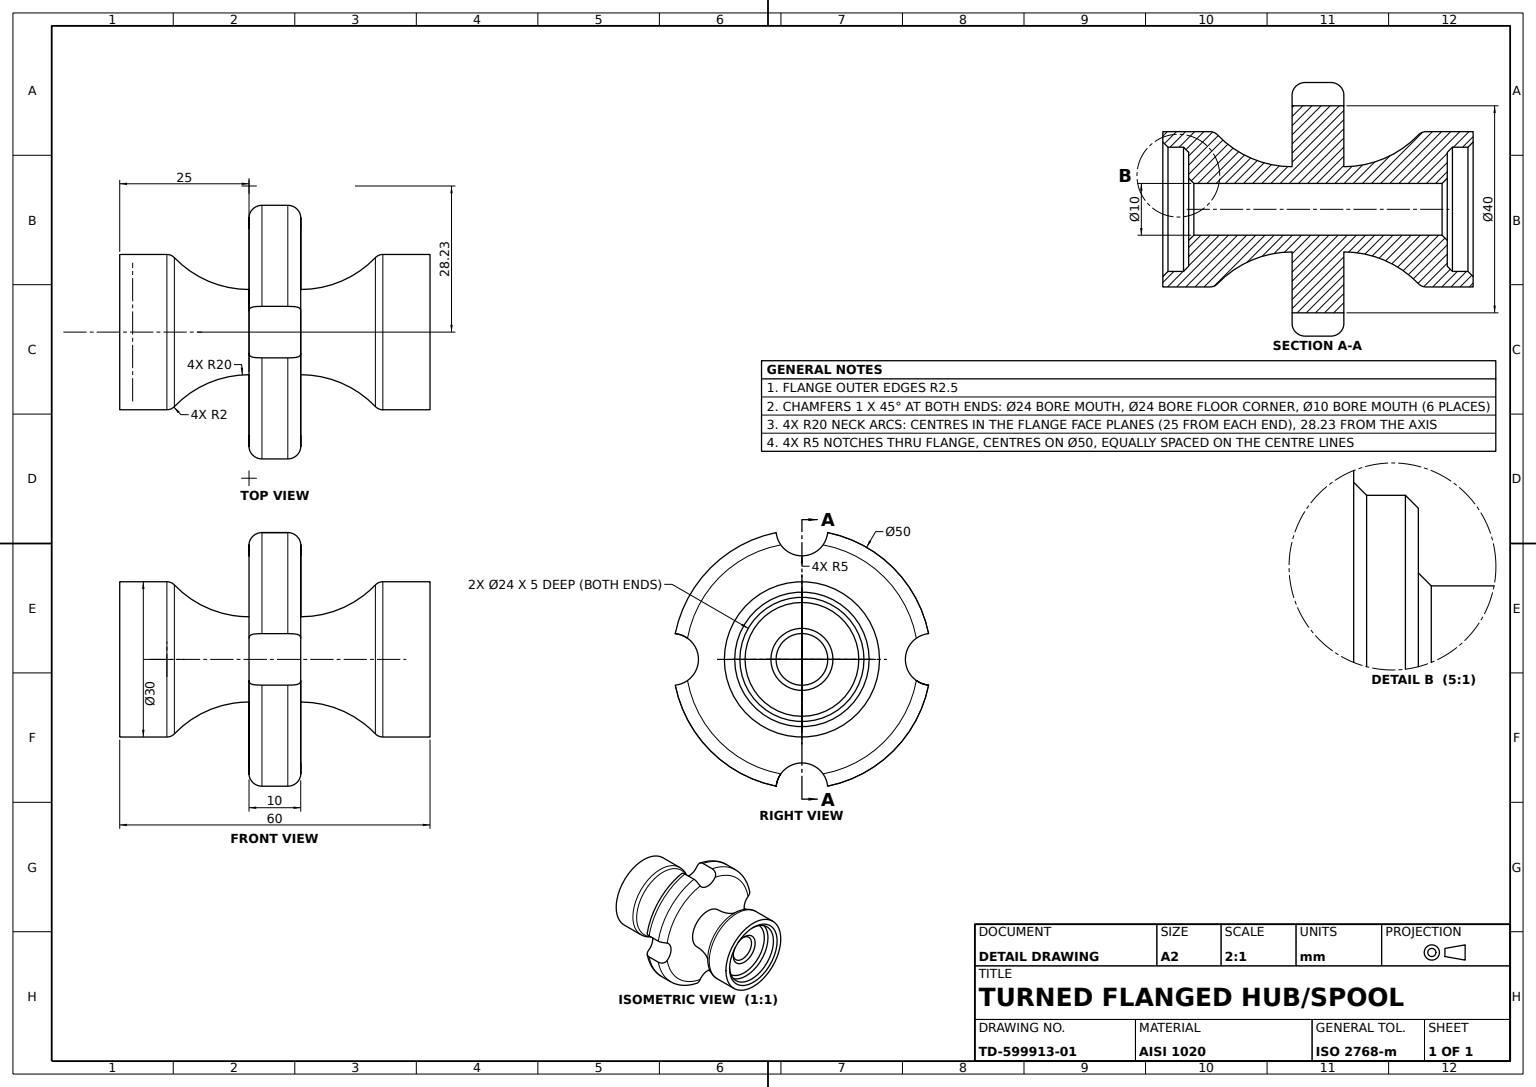
from build123d import *

# Parameters (mm, degrees)
FLANGE_FILLET_R2_5_R     = 2.5
FLANGE_NOTCHES_4X_REACH  = 51.749
FLANGE_NOTCH_SKETCH_R    = 5
EDGE_CHAMFER_1X45_A_SIZE = 1
EDGE_FILLET_R2_R         = 2
EDGE_CHAMFER_1X45_B_SIZE = 1


with BuildPart() as part:
    # Hub Profile Sketch → Hub Body Revolve (revolve)
    with BuildSketch(Plane.XY, mode=Mode.PRIVATE) as hub_body_revolve_sk:
        with BuildLine():
            Line((12, 0), (12, 5))
            Line((12, 5), (5, 5))
            Line((5, 5), (5, 55))
            Line((5, 55), (12, 55))
            Line((12, 55), (12, 60))
            Line((12, 60), (15, 60))
            Line((15, 60), (15, 50))
            ThreePointArc((15, 50), (10, 43.228756555), (8.228756555, 35))
            Line((8.228756555, 35), (25, 35))
            Line((25, 35), (25, 25))
            Line((25, 25), (8.228756555, 25))
            ThreePointArc((8.228756555, 25), (10, 16.771243445), (15, 10))
            Line((15, 10), (15, 0))
            Line((15, 0), (12, 0))
        make_face()
    revolve(hub_body_revolve_sk.sketch.rotate(Axis((0, 60, 0), (0, -1, 0)), 90), axis=Axis((0, 60, 0), (0, -1, 0)))

    # Flange Fillet R2.5
    flange_fillet_r2_5_edges = [part.edges().sort_by_distance(p)[0] for p in [
        (0, 25, -25),
        (0, 35, -25),
    ]]
    fillet(flange_fillet_r2_5_edges, radius=FLANGE_FILLET_R2_5_R)

    # Flange Notch Sketch → Flange Notches 4x (cut, up to next)
    with BuildSketch(Plane(origin=(0, 35, 0), x_dir=(1, 0, 0), z_dir=(0, 1, 0)), mode=Mode.PRIVATE) as flange_notches_4x_sk1:
        with Locations((0, 25)):
            Circle(FLANGE_NOTCH_SKETCH_R)
    flange_notches_4x_tool1 = extrude(flange_notches_4x_sk1.sketch, amount=-FLANGE_NOTCHES_4X_REACH, mode=Mode.PRIVATE) & part.part
    # Flange Notch Sketch → Flange Notches 4x (cut, up to next)
    with BuildSketch(Plane(origin=(0, 35, 0), x_dir=(1, 0, 0), z_dir=(0, 1, 0)), mode=Mode.PRIVATE) as flange_notches_4x_sk2:
        with Locations((25, 0)):
            Circle(FLANGE_NOTCH_SKETCH_R)
    flange_notches_4x_tool2 = extrude(flange_notches_4x_sk2.sketch, amount=-FLANGE_NOTCHES_4X_REACH, mode=Mode.PRIVATE) & part.part
    # Flange Notch Sketch → Flange Notches 4x (cut, up to next)
    with BuildSketch(Plane(origin=(0, 35, 0), x_dir=(1, 0, 0), z_dir=(0, 1, 0)), mode=Mode.PRIVATE) as flange_notches_4x_sk3:
        with Locations((0, -25)):
            Circle(FLANGE_NOTCH_SKETCH_R)
    flange_notches_4x_tool3 = extrude(flange_notches_4x_sk3.sketch, amount=-FLANGE_NOTCHES_4X_REACH, mode=Mode.PRIVATE) & part.part
    # Flange Notch Sketch → Flange Notches 4x (cut, up to next)
    with BuildSketch(Plane(origin=(0, 35, 0), x_dir=(1, 0, 0), z_dir=(0, 1, 0)), mode=Mode.PRIVATE) as flange_notches_4x_sk4:
        with Locations((-25, 0)):
            Circle(FLANGE_NOTCH_SKETCH_R)
    flange_notches_4x_tool4 = extrude(flange_notches_4x_sk4.sketch, amount=-FLANGE_NOTCHES_4X_REACH, mode=Mode.PRIVATE) & part.part
    add(flange_notches_4x_tool1.solids().sort_by_distance((0, 35, -25))[0], mode=Mode.SUBTRACT)
    add(flange_notches_4x_tool2.solids().sort_by_distance((25, 35, 0))[0], mode=Mode.SUBTRACT)
    add(flange_notches_4x_tool3.solids().sort_by_distance((0, 35, 25))[0], mode=Mode.SUBTRACT)
    add(flange_notches_4x_tool4.solids().sort_by_distance((-25, 35, 0))[0], mode=Mode.SUBTRACT)

    # Edge Chamfer 1x45 A
    edge_chamfer_1x45_a_edges = [part.edges().sort_by_distance(p)[0] for p in [
        (0, 60, -12),
        (0, 55, -5),
        (0, 5, -5),
        (0, 0, -12),
    ]]
    chamfer(edge_chamfer_1x45_a_edges, length=EDGE_CHAMFER_1X45_A_SIZE)

    # Edge Fillet R2
    edge_fillet_r2_edges = [part.edges().sort_by_distance(p)[0] for p in [
        (0, 10, -15),
        (0, 50, -15),
    ]]
    fillet(edge_fillet_r2_edges, radius=EDGE_FILLET_R2_R)

    # Edge Chamfer 1x45 B
    edge_chamfer_1x45_b_edges = [part.edges().sort_by_distance(p)[0] for p in [
        (0, 55, -12),
        (0, 5, -12),
    ]]
    chamfer(edge_chamfer_1x45_b_edges, length=EDGE_CHAMFER_1X45_B_SIZE)


solid = part.part
